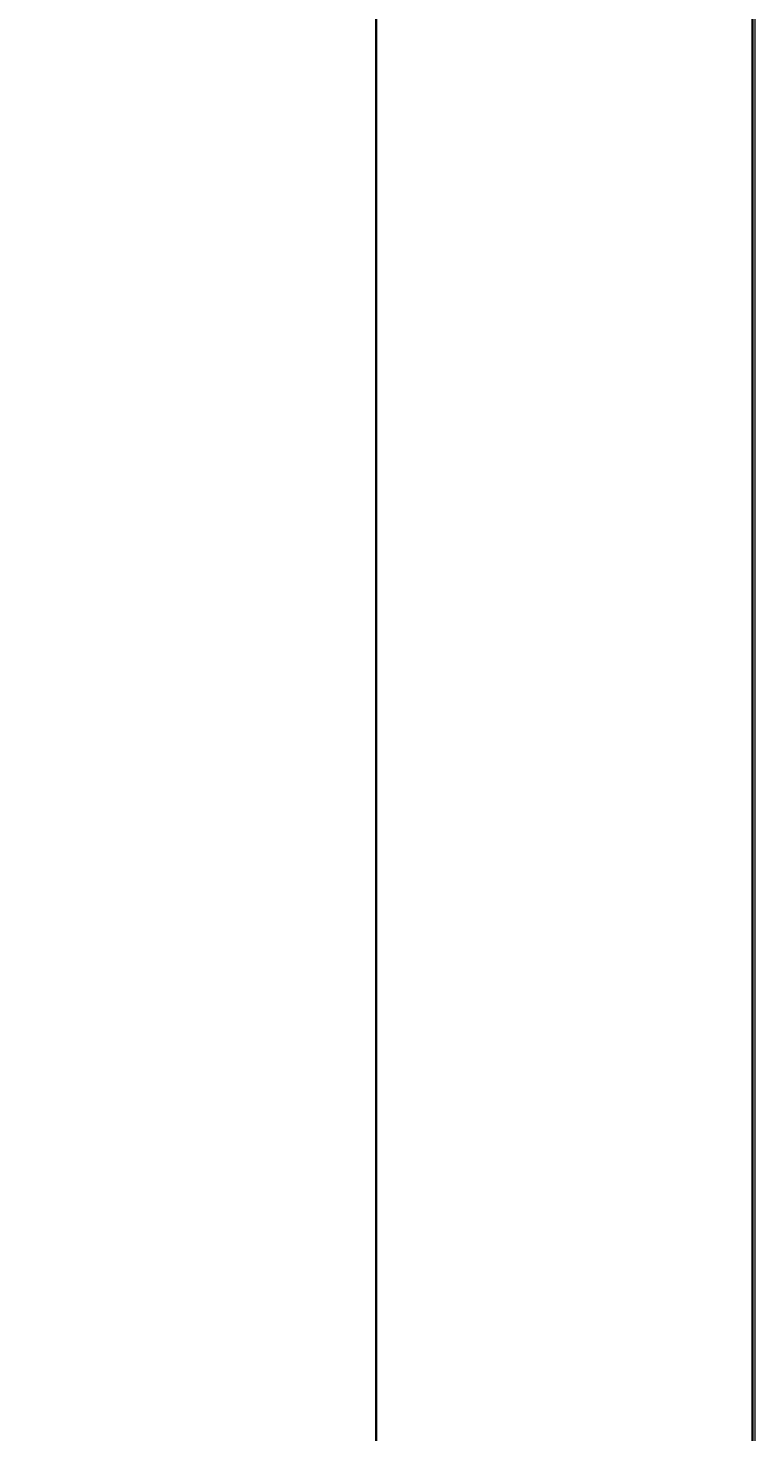
# Model space of a CAD drawing. Units: millimetres. Extents: x 27017497 to 27018854, y 7058029 to 7059154.
# Tile 7 of 91: x 27017605 to 27017623, y 7058166 to 7058200. Entities that reach past the tile are written whole.
import ezdxf

# ---------------------------------------------------------------- set-up
doc = ezdxf.new("R2010")
doc.units = ezdxf.units.MM
for name, color, linetype, lineweight in [('A-ANNO-DIMS', 2, 'Continuous', 18), ('A-FLOR-CASE', 8, 'Continuous', 20), ('A-WALL', 7, 'Continuous', 35)]:
    doc.layers.add(name, color=color, linetype=linetype, lineweight=lineweight)
doc.styles.get("Standard").update_dxf_attribs({"font": 'arial.ttf'})
doc.dimstyles.get("Standard").update_dxf_attribs({"dimtxt": 0.18, "dimasz": 0.18, "dimexe": 0.18, "dimexo": 0.0625, "dimgap": 0.09, "dimtad": 0, "dimtih": 1, "dimtoh": 1, "dimdec": 4, "dimzin": 0, "dimdsep": 46, "dimtxsty": 'Standard', "dimcen": 0.09, "dimadec": 0, "dimazin": 0, "dimtfac": 1, "dimtdec": 4, "dimtofl": 0, "dimtmove": 0, "dimatfit": 3, "dimfxl": 1, "dimtolj": 1, "dimtzin": 0, "dimarcsym": 0})

# ---------------------------------------------------------------- blocks, each defined once
blk = doc.blocks.new('WARDROBE-HANGING')
blk.add_line((0, 0), (65.212, 0))
blk = doc.blocks.new('*D47')
at = {"layer": 'A-ANNO-DIMS', "color": 0, "lineweight": -2, "transparency": 16777216}
for p, q in [((27017561.166, 7058294.35), (27017561.166, 7058028.6)), ((27018790.606, 7058294.35), (27018790.606, 7058028.6)), ((27017561.346, 7058028.78), (27018175.431, 7058028.78)), ((27018790.426, 7058028.78), (27018176.341, 7058028.78))]:
    blk.add_line(p, q, dxfattribs=at)
at = {"layer": 'A-ANNO-DIMS', "color": 0, "transparency": 16777216}
for points in [[(27017561.346, 7058028.81), (27017561.346, 7058028.75), (27017561.166, 7058028.78)], [(27018790.426, 7058028.81), (27018790.426, 7058028.75), (27018790.606, 7058028.78)]]:
    blk.add_solid(points, dxfattribs=at)
at = {"layer": 'Defpoints', "color": 0, "transparency": 16777216}
for p in [(27017561.166, 7058294.412), (27018790.606, 7058294.412), (27018790.606, 7058028.78)]:
    blk.add_point(p, dxfattribs=at)
at = {"layer": 'A-ANNO-DIMS', "color": 0, "transparency": 16777216, "insert": (27018175.886, 7058028.78), "char_height": 0.18, "attachment_point": 5}
blk.add_mtext('\\A1;1229.4', dxfattribs=at)
blk = doc.blocks.new('*D48')
at = {"layer": 'A-ANNO-DIMS', "color": 0, "lineweight": -2, "transparency": 16777216}
for p, q in [((27018463.498, 7058622.912), (27017497.536, 7058622.912)), ((27017497.716, 7058622.732), (27017497.716, 7058357.753)), ((27017497.716, 7058092.41), (27017497.716, 7058357.389)), ((27018555.129, 7058092.23), (27017497.536, 7058092.23))]:
    blk.add_line(p, q, dxfattribs=at)
at = {"layer": 'A-ANNO-DIMS', "color": 0, "transparency": 16777216}
for points in [[(27017497.686, 7058622.732), (27017497.746, 7058622.732), (27017497.716, 7058622.912)], [(27017497.686, 7058092.41), (27017497.746, 7058092.41), (27017497.716, 7058092.23)]]:
    blk.add_solid(points, dxfattribs=at)
at = {"layer": 'Defpoints', "color": 0, "transparency": 16777216}
for p in [(27018463.561, 7058622.912), (27017497.716, 7058092.23), (27018555.192, 7058092.23)]:
    blk.add_point(p, dxfattribs=at)
at = {"layer": 'A-ANNO-DIMS', "color": 0, "transparency": 16777216, "insert": (27017497.716, 7058357.571), "char_height": 0.18, "attachment_point": 5}
blk.add_mtext('\\A1;530.7', dxfattribs=at)

msp = doc.modelspace()

# ---------------------------------------------------------------- linework, layer by layer
at = {"layer": 'A-WALL'}
for p, q in [((27017613.666, 7058294.412), (27017613.666, 7058132.912)), ((27017622.666, 7058294.412), (27017622.666, 7058141.912))]:
    msp.add_line(p, q, dxfattribs=at)

# ---------------------------------------------------------------- block references
at = {"layer": 'A-FLOR-CASE', "rotation": 270}
msp.add_blockref('WARDROBE-HANGING', (27017622.724, 7058207.1), dxfattribs=at)

# ---------------------------------------------------------------- dimensions: what is measured, and where the dimension line sits
at = {"layer": 'A-ANNO-DIMS'}
dim = msp.add_linear_dim(base=(27017497.716, 7058092.23), p1=(27018463.561, 7058622.912), p2=(27018555.192, 7058092.23), angle=90, dimstyle='Standard', override={"dimdec": 1, "dimlfac": 1, "dimrnd": 0, "dimzin": 0, "dimdsep": 46, "dimlunit": 2}, dxfattribs=at)
dim.commit()
dim.dimension.update_dxf_attribs({"geometry": '*D48', "text_midpoint": (27017497.716, 7058357.571)})
dim = msp.add_linear_dim(base=(27018790.606, 7058028.78), p1=(27017561.166, 7058294.412), p2=(27018790.606, 7058294.412), dimstyle='Standard', override={"dimdec": 1, "dimlfac": 1, "dimrnd": 0, "dimzin": 0, "dimdsep": 46, "dimlunit": 2}, dxfattribs=at)
dim.commit()
dim.dimension.update_dxf_attribs({"geometry": '*D47', "text_midpoint": (27018175.886, 7058028.78)})

doc.saveas('drawing.dxf')
